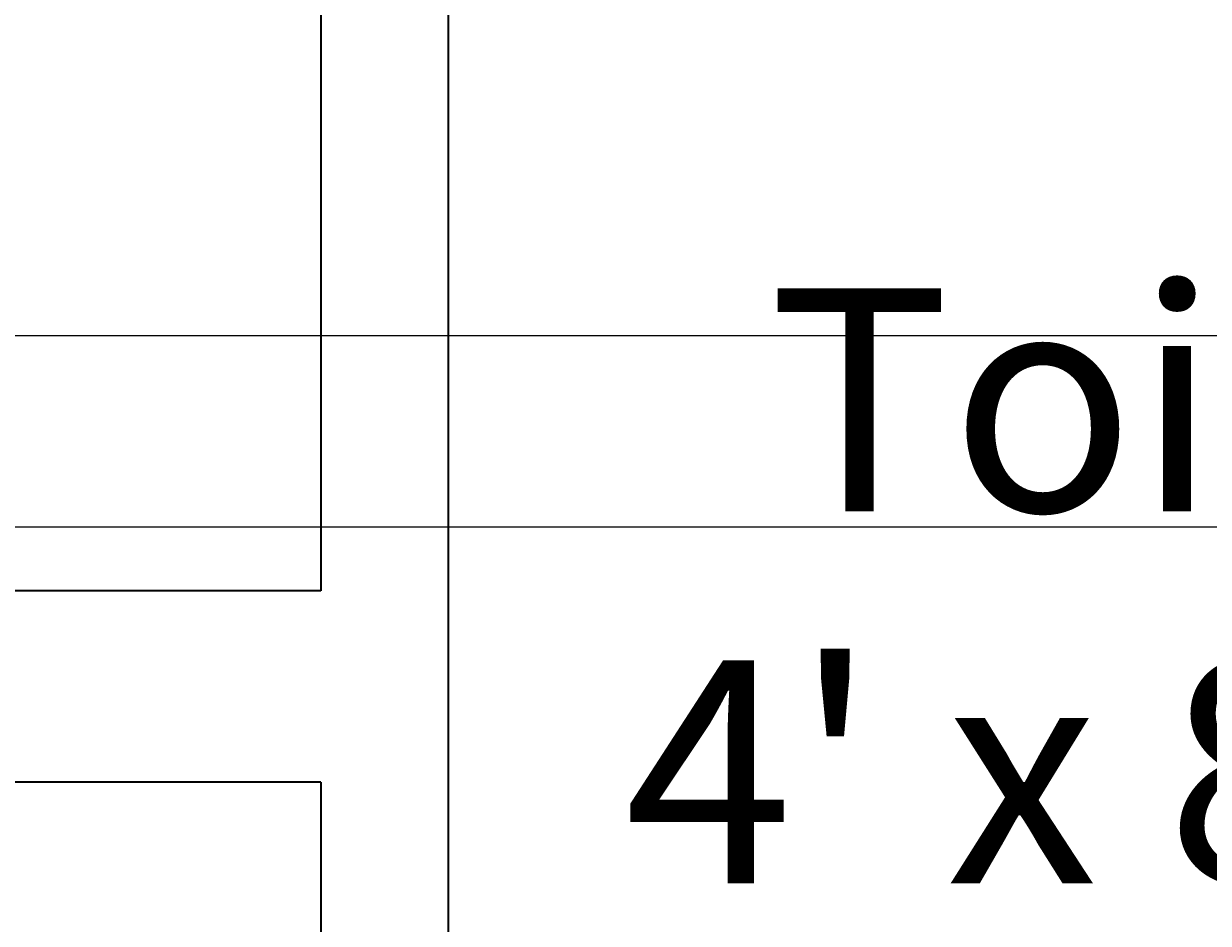
# Model space of a CAD drawing. Units: feet. Extents: x 105 to 1094, y -88 to 588.
# Tile 12 of 59: x 361 to 399, y 194 to 222. Entities that reach past the tile are written whole.
import ezdxf

# ---------------------------------------------------------------- set-up
doc = ezdxf.new("R2010")
doc.units = ezdxf.units.FT
doc.header["$MEASUREMENT"] = 0
for name, color, linetype, lineweight in [('A-ANNO-DIMS', 2, 'Continuous', 18), ('A-AREA-IDEN', 7, 'Continuous', 18), ('A-WALL', 7, 'Continuous', 35)]:
    doc.layers.add(name, color=color, linetype=linetype, lineweight=lineweight)
doc.styles.get("Standard").update_dxf_attribs({"font": 'arial.ttf'})
doc.dimstyles.get("Standard").update_dxf_attribs({"dimtxt": 0.18, "dimasz": 0.18, "dimexe": 0.18, "dimexo": 0.0625, "dimgap": 0.09, "dimtad": 0, "dimtih": 1, "dimtoh": 1, "dimdec": 4, "dimzin": 0, "dimdsep": 46, "dimtxsty": 'Standard', "dimcen": 0.09, "dimadec": 0, "dimazin": 0, "dimtfac": 1, "dimtdec": 4, "dimtofl": 0, "dimtmove": 0, "dimatfit": 3, "dimfxl": 1, "dimtolj": 1, "dimtzin": 0, "dimarcsym": 0})

# ---------------------------------------------------------------- blocks, each defined once
blk = doc.blocks.new('*D20')
at = {"layer": 'A-ANNO-DIMS', "color": 0, "lineweight": -2, "transparency": 16777216}
for p, q in [((150.688, 276.019), (150.688, -88.149)), ((1048.688, 276.019), (1048.688, -88.149)), ((150.868, -87.969), (599.399, -87.969)), ((1048.508, -87.969), (599.977, -87.969))]:
    blk.add_line(p, q, dxfattribs=at)
at = {"layer": 'A-ANNO-DIMS', "color": 0, "transparency": 16777216}
for points in [[(150.868, -87.939), (150.868, -87.999), (150.688, -87.969)], [(1048.508, -87.939), (1048.508, -87.999), (1048.688, -87.969)]]:
    blk.add_solid(points, dxfattribs=at)
at = {"layer": 'Defpoints', "color": 0, "transparency": 16777216}
for p in [(150.688, 276.081), (1048.688, 276.081), (1048.688, -87.969)]:
    blk.add_point(p, dxfattribs=at)
at = {"layer": 'A-ANNO-DIMS', "color": 0, "transparency": 16777216, "insert": (599.688, -87.969), "char_height": 0.18, "attachment_point": 5}
blk.add_mtext('\\A1;898', dxfattribs=at)
blk = doc.blocks.new('*D21')
at = {"layer": 'A-ANNO-DIMS', "color": 0, "lineweight": -2, "transparency": 16777216}
for p, q in [((849.626, 543.081), (105.458, 543.081)), ((105.638, 542.901), (105.638, 250.263)), ((105.638, -42.739), (105.638, 249.899)), ((849.626, -42.919), (105.458, -42.919))]:
    blk.add_line(p, q, dxfattribs=at)
at = {"layer": 'A-ANNO-DIMS', "color": 0, "transparency": 16777216}
for points in [[(105.608, 542.901), (105.668, 542.901), (105.638, 543.081)], [(105.608, -42.739), (105.668, -42.739), (105.638, -42.919)]]:
    blk.add_solid(points, dxfattribs=at)
at = {"layer": 'Defpoints', "color": 0, "transparency": 16777216}
for p in [(105.638, 543.081), (849.688, 543.081), (849.688, -42.919)]:
    blk.add_point(p, dxfattribs=at)
at = {"layer": 'A-ANNO-DIMS', "color": 0, "transparency": 16777216, "insert": (105.638, 250.081), "char_height": 0.18, "attachment_point": 5}
blk.add_mtext('\\A1;586', dxfattribs=at)
blk = doc.blocks.new('*D36')
at = {"layer": 'A-ANNO-DIMS', "color": 0, "lineweight": -2, "transparency": 16777216}
for p, q in [((547.235, 248.081), (105.458, 248.081)), ((105.638, 247.901), (105.638, 230.263)), ((105.638, 212.261), (105.638, 229.899)), ((546.626, 212.081), (105.458, 212.081))]:
    blk.add_line(p, q, dxfattribs=at)
at = {"layer": 'A-ANNO-DIMS', "color": 0, "transparency": 16777216}
for points in [[(105.608, 247.901), (105.668, 247.901), (105.638, 248.081)], [(105.608, 212.261), (105.668, 212.261), (105.638, 212.081)]]:
    blk.add_solid(points, dxfattribs=at)
at = {"layer": 'Defpoints', "color": 0, "transparency": 16777216}
for p in [(105.638, 248.081), (547.298, 248.081), (546.688, 212.081)]:
    blk.add_point(p, dxfattribs=at)
at = {"layer": 'A-ANNO-DIMS', "color": 0, "transparency": 16777216, "insert": (105.638, 230.081), "char_height": 0.18, "attachment_point": 5}
blk.add_mtext('\\A1;36', dxfattribs=at)
blk = doc.blocks.new('*D39')
at = {"layer": 'A-ANNO-DIMS', "color": 0, "lineweight": -2, "transparency": 16777216}
for p, q in [((294.688, 204.144), (294.688, 588.311)), ((370.688, 204.144), (370.688, 588.311)), ((294.868, 588.131), (332.47, 588.131)), ((370.508, 588.131), (332.906, 588.131))]:
    blk.add_line(p, q, dxfattribs=at)
at = {"layer": 'A-ANNO-DIMS', "color": 0, "transparency": 16777216}
for points in [[(294.868, 588.161), (294.868, 588.101), (294.688, 588.131)], [(370.508, 588.161), (370.508, 588.101), (370.688, 588.131)]]:
    blk.add_solid(points, dxfattribs=at)
at = {"layer": 'Defpoints', "color": 0, "transparency": 16777216}
for p in [(370.688, 588.131), (294.688, 204.081), (370.688, 204.081)]:
    blk.add_point(p, dxfattribs=at)
at = {"layer": 'A-ANNO-DIMS', "color": 0, "transparency": 16777216, "insert": (332.688, 588.131), "char_height": 0.18, "attachment_point": 5}
blk.add_mtext('\\A1;76', dxfattribs=at)
blk = doc.blocks.new('*D46')
at = {"layer": 'A-ANNO-DIMS', "color": 0, "lineweight": -2, "transparency": 16777216}
for p, q in [((580.626, 206.081), (105.458, 206.081)), ((105.638, 205.901), (105.638, 173.263)), ((105.638, 140.261), (105.638, 172.899)), ((580.626, 140.081), (105.458, 140.081))]:
    blk.add_line(p, q, dxfattribs=at)
at = {"layer": 'A-ANNO-DIMS', "color": 0, "transparency": 16777216}
for points in [[(105.608, 205.901), (105.668, 205.901), (105.638, 206.081)], [(105.608, 140.261), (105.668, 140.261), (105.638, 140.081)]]:
    blk.add_solid(points, dxfattribs=at)
at = {"layer": 'Defpoints', "color": 0, "transparency": 16777216}
for p in [(580.688, 206.081), (105.638, 140.081), (580.688, 140.081)]:
    blk.add_point(p, dxfattribs=at)
at = {"layer": 'A-ANNO-DIMS', "color": 0, "transparency": 16777216, "insert": (105.638, 173.081), "char_height": 0.18, "attachment_point": 5}
blk.add_mtext('\\A1;66', dxfattribs=at)

msp = doc.modelspace()

# ---------------------------------------------------------------- linework, layer by layer
at = {"layer": 'A-WALL'}
for p, q in [((370.6883, 252.0812), (370.6883, 204.0812)), ((374.6883, 248.0812), (374.6883, 146.0812)), ((370.6883, 204.0812), (294.6883, 204.0812)), ((370.6883, 198.0812), (292.6883, 198.0812)), ((370.6883, 198.0812), (370.6883, 150.0812))]:
    msp.add_line(p, q, dxfattribs=at)

# ---------------------------------------------------------------- texts
at = {"layer": 'A-AREA-IDEN', "insert": (446.7646, 194.9029), "char_height": 7, "attachment_point": 9}
msp.add_mtext_dynamic_manual_height_columns('\\pxqc;Toilet \\P4\' x 8\'2"', width=98.34246, gutter_width=1, heights=[0], dxfattribs=at)

# ---------------------------------------------------------------- dimensions: what is measured, and where the dimension line sits
at = {"layer": 'A-ANNO-DIMS'}
for base, p1, p2, picture, middle in [((370.6883, 588.1312), (294.6883, 204.0812), (370.6883, 204.0812), '*D39', (332.6883, 588.1312)), ((1048.6883, -87.9688), (150.6883, 276.0812), (1048.6883, 276.0812), '*D20', (599.6883, -87.9688))]:
    dim = msp.add_linear_dim(base=base, p1=p1, p2=p2, dimstyle='Standard', override={"dimdec": 0, "dimlfac": 1, "dimrnd": 0, "dimzin": 0, "dimdsep": 46, "dimlunit": 2}, dxfattribs=at)
    dim.commit()
    dim.dimension.update_dxf_attribs({"geometry": picture, "text_midpoint": middle})
for base, p1, p2, picture, middle in [((105.6383, 543.0812), (849.6883, -42.9188), (849.6883, 543.0812), '*D21', (105.6383, 250.0812)), ((105.6383, 248.0812), (546.6883, 212.0812), (547.2975, 248.0812), '*D36', (105.6383, 230.0812)), ((105.6383, 140.0812), (580.6883, 206.0812), (580.6883, 140.0812), '*D46', (105.6383, 173.0812))]:
    dim = msp.add_linear_dim(base=base, p1=p1, p2=p2, angle=90, dimstyle='Standard', override={"dimdec": 0, "dimlfac": 1, "dimrnd": 0, "dimzin": 0, "dimdsep": 46, "dimlunit": 2}, dxfattribs=at)
    dim.commit()
    dim.dimension.update_dxf_attribs({"geometry": picture, "text_midpoint": middle})

doc.saveas('drawing.dxf')
